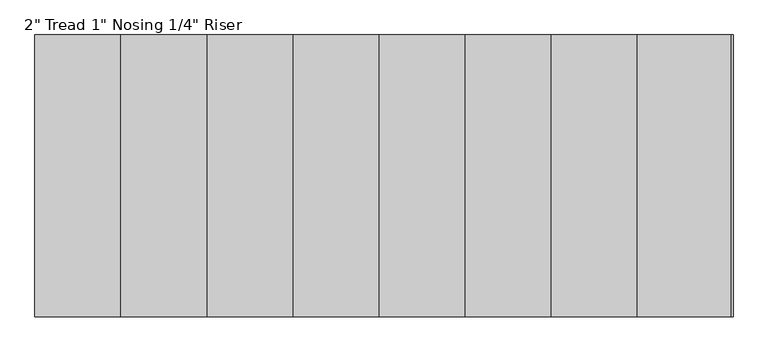
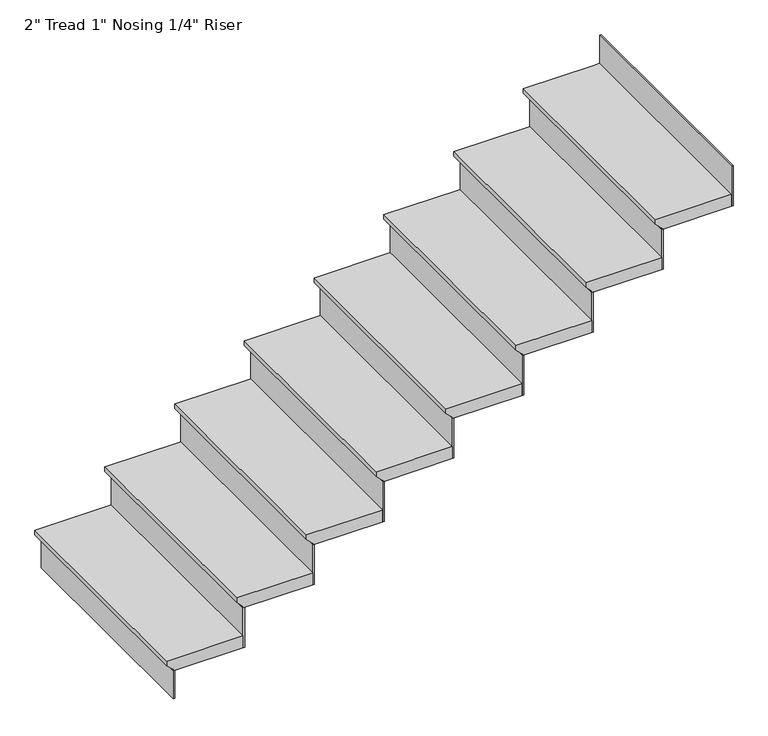
"""IFC4 building model written with IfcOpenShell, lengths in millimetres: stair flight geometry."""

from ifc_helpers import new_model, si_unit, origin, place, context, project, spatial, faceted_brep, source, transform, mapped, element, save


def stair_flight_1fa62499(model_context):
    return source(origin(), model_context, "Body", "Brep", [
        faceted_brep([(-3925.4851125, 1242.1395264, 150.2833333), (-3925.4851125, 1242.1395264, 169.3333333), (-3925.4851125, 2156.5395264, 169.3333333), (-3925.4851125, 2156.5395264, 150.2833333), (-3900.0851125, 1242.1395264, 124.8833333), (-3900.0851125, 2156.5395264, 124.8833333), (-3620.6851125, 1242.1395264, 169.3333333), (-3620.6851125, 2156.5395264, 169.3333333), (-3900.0851125, 2156.5395264, 118.5333333), (-3620.6851125, 2156.5395264, 118.5333333), (-3620.6851125, 1242.1395264, 118.5333333), (-3900.0851125, 1242.1395264, 118.5333333)], [[[0, 1, 2, 3]], [[4, 0, 3, 5]], [[2, 1, 6, 7]], [[8, 9, 10, 11]], [[2, 7, 9, 8, 5, 3]], [[8, 11, 4, 5]], [[6, 1, 0, 4, 11, 10]], [[7, 6, 10, 9]]]),
        faceted_brep([(-3900.0851125, 1242.1395264, 118.5333333), (-3900.0851125, 1242.1395264, 0.0), (-3893.7351125, 1242.1395264, 0.0), (-3893.7351125, 1242.1395264, 118.5333333), (-3900.0851125, 2156.5395264, 118.5333333), (-3893.7351125, 2156.5395264, 118.5333333), (-3893.7351125, 2156.5395264, 0.0), (-3900.0851125, 2156.5395264, 0.0)], [[[0, 1, 2, 3]], [[4, 5, 6, 7]], [[1, 0, 4, 7]], [[2, 1, 7, 6]], [[3, 2, 6, 5]], [[0, 3, 5, 4]]]),
        faceted_brep([(-3620.6851125, 1242.1395264, 287.8666667), (-3620.6851125, 1242.1395264, 118.5333333), (-3614.3351125, 1242.1395264, 118.5333333), (-3614.3351125, 1242.1395264, 287.8666667), (-3620.6851125, 2156.5395264, 287.8666667), (-3614.3351125, 2156.5395264, 287.8666667), (-3614.3351125, 2156.5395264, 118.5333333), (-3620.6851125, 2156.5395264, 118.5333333)], [[[0, 1, 2, 3]], [[4, 5, 6, 7]], [[1, 0, 4, 7]], [[2, 1, 7, 6]], [[3, 2, 6, 5]], [[0, 3, 5, 4]]]),
        faceted_brep([(-3646.0851125, 2156.5395264, 338.6666667), (-3646.0851125, 1242.1395264, 338.6666667), (-3341.2851125, 1242.1395264, 338.6666667), (-3341.2851125, 2156.5395264, 338.6666667), (-3620.6851125, 2156.5395264, 287.8666667), (-3341.2851125, 2156.5395264, 287.8666667), (-3341.2851125, 1242.1395264, 287.8666667), (-3620.6851125, 1242.1395264, 287.8666667), (-3620.6851125, 2156.5395264, 294.2166667), (-3646.0851125, 2156.5395264, 319.6166667), (-3620.6851125, 1242.1395264, 294.2166667), (-3646.0851125, 1242.1395264, 319.6166667)], [[[0, 1, 2, 3]], [[4, 5, 6, 7]], [[0, 3, 5, 4, 8, 9]], [[4, 7, 10, 8]], [[2, 1, 11, 10, 7, 6]], [[3, 2, 6, 5]], [[11, 1, 0, 9]], [[10, 11, 9, 8]]]),
        faceted_brep([(-3341.2851125, 1242.1395264, 457.2), (-3341.2851125, 1242.1395264, 287.8666667), (-3334.9351125, 1242.1395264, 287.8666667), (-3334.9351125, 1242.1395264, 457.2), (-3341.2851125, 2156.5395264, 457.2), (-3334.9351125, 2156.5395264, 457.2), (-3334.9351125, 2156.5395264, 287.8666667), (-3341.2851125, 2156.5395264, 287.8666667)], [[[0, 1, 2, 3]], [[4, 5, 6, 7]], [[1, 0, 4, 7]], [[2, 1, 7, 6]], [[3, 2, 6, 5]], [[0, 3, 5, 4]]]),
        faceted_brep([(-3366.6851125, 2156.5395264, 508.0), (-3366.6851125, 1242.1395264, 508.0), (-3061.8851125, 1242.1395264, 508.0), (-3061.8851125, 2156.5395264, 508.0), (-3341.2851125, 2156.5395264, 457.2), (-3061.8851125, 2156.5395264, 457.2), (-3061.8851125, 1242.1395264, 457.2), (-3341.2851125, 1242.1395264, 457.2), (-3341.2851125, 2156.5395264, 463.55), (-3366.6851125, 2156.5395264, 488.95), (-3341.2851125, 1242.1395264, 463.55), (-3366.6851125, 1242.1395264, 488.95)], [[[0, 1, 2, 3]], [[4, 5, 6, 7]], [[0, 3, 5, 4, 8, 9]], [[4, 7, 10, 8]], [[2, 1, 11, 10, 7, 6]], [[3, 2, 6, 5]], [[11, 1, 0, 9]], [[10, 11, 9, 8]]]),
        faceted_brep([(-3061.8851125, 1242.1395264, 626.5333333), (-3061.8851125, 1242.1395264, 457.2), (-3055.5351125, 1242.1395264, 457.2), (-3055.5351125, 1242.1395264, 626.5333333), (-3061.8851125, 2156.5395264, 626.5333333), (-3055.5351125, 2156.5395264, 626.5333333), (-3055.5351125, 2156.5395264, 457.2), (-3061.8851125, 2156.5395264, 457.2)], [[[0, 1, 2, 3]], [[4, 5, 6, 7]], [[1, 0, 4, 7]], [[2, 1, 7, 6]], [[3, 2, 6, 5]], [[0, 3, 5, 4]]]),
        faceted_brep([(-3087.2851125, 2156.5395264, 677.3333333), (-3087.2851125, 1242.1395264, 677.3333333), (-2782.4851125, 1242.1395264, 677.3333333), (-2782.4851125, 2156.5395264, 677.3333333), (-3061.8851125, 2156.5395264, 626.5333333), (-2782.4851125, 2156.5395264, 626.5333333), (-2782.4851125, 1242.1395264, 626.5333333), (-3061.8851125, 1242.1395264, 626.5333333), (-3061.8851125, 2156.5395264, 632.8833333), (-3087.2851125, 2156.5395264, 658.2833333), (-3061.8851125, 1242.1395264, 632.8833333), (-3087.2851125, 1242.1395264, 658.2833333)], [[[0, 1, 2, 3]], [[4, 5, 6, 7]], [[0, 3, 5, 4, 8, 9]], [[4, 7, 10, 8]], [[2, 1, 11, 10, 7, 6]], [[3, 2, 6, 5]], [[11, 1, 0, 9]], [[10, 11, 9, 8]]]),
        faceted_brep([(-2782.4851125, 1242.1395264, 795.8666667), (-2782.4851125, 1242.1395264, 626.5333333), (-2776.1351125, 1242.1395264, 626.5333333), (-2776.1351125, 1242.1395264, 795.8666667), (-2782.4851125, 2156.5395264, 795.8666667), (-2776.1351125, 2156.5395264, 795.8666667), (-2776.1351125, 2156.5395264, 626.5333333), (-2782.4851125, 2156.5395264, 626.5333333)], [[[0, 1, 2, 3]], [[4, 5, 6, 7]], [[1, 0, 4, 7]], [[2, 1, 7, 6]], [[3, 2, 6, 5]], [[0, 3, 5, 4]]]),
        faceted_brep([(-2807.8851125, 2156.5395264, 846.6666667), (-2807.8851125, 1242.1395264, 846.6666667), (-2503.0851125, 1242.1395264, 846.6666667), (-2503.0851125, 2156.5395264, 846.6666667), (-2782.4851125, 2156.5395264, 795.8666667), (-2503.0851125, 2156.5395264, 795.8666667), (-2503.0851125, 1242.1395264, 795.8666667), (-2782.4851125, 1242.1395264, 795.8666667), (-2782.4851125, 2156.5395264, 802.2166667), (-2807.8851125, 2156.5395264, 827.6166667), (-2782.4851125, 1242.1395264, 802.2166667), (-2807.8851125, 1242.1395264, 827.6166667)], [[[0, 1, 2, 3]], [[4, 5, 6, 7]], [[0, 3, 5, 4, 8, 9]], [[4, 7, 10, 8]], [[2, 1, 11, 10, 7, 6]], [[3, 2, 6, 5]], [[11, 1, 0, 9]], [[10, 11, 9, 8]]]),
        faceted_brep([(-2503.0851125, 1242.1395264, 965.2), (-2503.0851125, 1242.1395264, 795.8666667), (-2496.7351125, 1242.1395264, 795.8666667), (-2496.7351125, 1242.1395264, 965.2), (-2503.0851125, 2156.5395264, 965.2), (-2496.7351125, 2156.5395264, 965.2), (-2496.7351125, 2156.5395264, 795.8666667), (-2503.0851125, 2156.5395264, 795.8666667)], [[[0, 1, 2, 3]], [[4, 5, 6, 7]], [[1, 0, 4, 7]], [[2, 1, 7, 6]], [[3, 2, 6, 5]], [[0, 3, 5, 4]]]),
        faceted_brep([(-2528.4851125, 2156.5395264, 1016.0), (-2528.4851125, 1242.1395264, 1016.0), (-2223.6851125, 1242.1395264, 1016.0), (-2223.6851125, 2156.5395264, 1016.0), (-2503.0851125, 2156.5395264, 965.2), (-2223.6851125, 2156.5395264, 965.2), (-2223.6851125, 1242.1395264, 965.2), (-2503.0851125, 1242.1395264, 965.2), (-2503.0851125, 2156.5395264, 971.55), (-2528.4851125, 2156.5395264, 996.95), (-2503.0851125, 1242.1395264, 971.55), (-2528.4851125, 1242.1395264, 996.95)], [[[0, 1, 2, 3]], [[4, 5, 6, 7]], [[0, 3, 5, 4, 8, 9]], [[4, 7, 10, 8]], [[2, 1, 11, 10, 7, 6]], [[3, 2, 6, 5]], [[11, 1, 0, 9]], [[10, 11, 9, 8]]]),
        faceted_brep([(-2223.6851125, 1242.1395264, 1134.5333333), (-2223.6851125, 1242.1395264, 965.2), (-2217.3351125, 1242.1395264, 965.2), (-2217.3351125, 1242.1395264, 1134.5333333), (-2223.6851125, 2156.5395264, 1134.5333333), (-2217.3351125, 2156.5395264, 1134.5333333), (-2217.3351125, 2156.5395264, 965.2), (-2223.6851125, 2156.5395264, 965.2)], [[[0, 1, 2, 3]], [[4, 5, 6, 7]], [[1, 0, 4, 7]], [[2, 1, 7, 6]], [[3, 2, 6, 5]], [[0, 3, 5, 4]]]),
        faceted_brep([(-2249.0851125, 2156.5395264, 1185.3333333), (-2249.0851125, 1242.1395264, 1185.3333333), (-1944.2851125, 1242.1395264, 1185.3333333), (-1944.2851125, 2156.5395264, 1185.3333333), (-2223.6851125, 2156.5395264, 1134.5333333), (-1944.2851125, 2156.5395264, 1134.5333333), (-1944.2851125, 1242.1395264, 1134.5333333), (-2223.6851125, 1242.1395264, 1134.5333333), (-2223.6851125, 2156.5395264, 1140.8833333), (-2249.0851125, 2156.5395264, 1166.2833333), (-2223.6851125, 1242.1395264, 1140.8833333), (-2249.0851125, 1242.1395264, 1166.2833333)], [[[0, 1, 2, 3]], [[4, 5, 6, 7]], [[0, 3, 5, 4, 8, 9]], [[4, 7, 10, 8]], [[2, 1, 11, 10, 7, 6]], [[3, 2, 6, 5]], [[11, 1, 0, 9]], [[10, 11, 9, 8]]]),
        faceted_brep([(-1664.8851125, 1242.1395264, 1473.2), (-1664.8851125, 1242.1395264, 1303.8666667), (-1658.5351125, 1242.1395264, 1303.8666667), (-1658.5351125, 1242.1395264, 1473.2), (-1664.8851125, 2156.5395264, 1473.2), (-1658.5351125, 2156.5395264, 1473.2), (-1658.5351125, 2156.5395264, 1303.8666667), (-1664.8851125, 2156.5395264, 1303.8666667)], [[[0, 1, 2, 3]], [[4, 5, 6, 7]], [[1, 0, 4, 7]], [[2, 1, 7, 6]], [[3, 2, 6, 5]], [[0, 3, 5, 4]]]),
        faceted_brep([(-1944.2851125, 1242.1395264, 1303.8666667), (-1944.2851125, 1242.1395264, 1134.5333333), (-1937.9351125, 1242.1395264, 1134.5333333), (-1937.9351125, 1242.1395264, 1303.8666667), (-1944.2851125, 2156.5395264, 1303.8666667), (-1937.9351125, 2156.5395264, 1303.8666667), (-1937.9351125, 2156.5395264, 1134.5333333), (-1944.2851125, 2156.5395264, 1134.5333333)], [[[0, 1, 2, 3]], [[4, 5, 6, 7]], [[1, 0, 4, 7]], [[2, 1, 7, 6]], [[3, 2, 6, 5]], [[0, 3, 5, 4]]]),
        faceted_brep([(-1664.8851125, 2156.5395264, 1354.6666667), (-1690.2851125, 2156.5395264, 1354.6666667), (-1969.6851125, 2156.5395264, 1354.6666667), (-1969.6851125, 1242.1395264, 1354.6666667), (-1664.8851125, 1242.1395264, 1354.6666667), (-1690.2851125, 2156.5395264, 1303.8666667), (-1664.8851125, 2156.5395264, 1303.8666667), (-1664.8851125, 1242.1395264, 1303.8666667), (-1944.2851125, 1242.1395264, 1303.8666667), (-1944.2851125, 2156.5395264, 1303.8666667), (-1944.2851125, 2156.5395264, 1310.2166667), (-1969.6851125, 2156.5395264, 1335.6166667), (-1944.2851125, 1242.1395264, 1310.2166667), (-1969.6851125, 1242.1395264, 1335.6166667)], [[[0, 1, 2, 3, 4]], [[5, 6, 7, 8, 9]], [[1, 0, 6, 5]], [[2, 1, 5, 9, 10, 11]], [[9, 8, 12, 10]], [[4, 3, 13, 12, 8, 7]], [[0, 4, 7, 6]], [[13, 3, 2, 11]], [[12, 13, 11, 10]]]),
    ])


if __name__ == "__main__":
    model = new_model("IFC4")
    model_context = context("Model", 3, world=origin())
    ifc_project = project(units=[si_unit("LENGTHUNIT", "METRE", prefix="MILLI")], contexts=[model_context])
    site = spatial("IfcSite", under=ifc_project)
    building = spatial("IfcBuilding", under=site)
    placement = place(None, origin())
    stair_flight_shape = stair_flight_1fa62499(model_context)
    element("IfcStairFlight", 1, ObjectType="2\" Tread 1\" Nosing 1/4\" Riser", at=placement, inside=building, context=model_context, shape_type="MappedRepresentation", body=[
        mapped(stair_flight_shape, transform((0.0, 0.0, 0.0), x_axis=(1.0, 0.0, 0.0), y_axis=(0.0, 1.0, 0.0), z_axis=(0.0, 0.0, 1.0))),
    ])
    save(model, "model.ifc")
